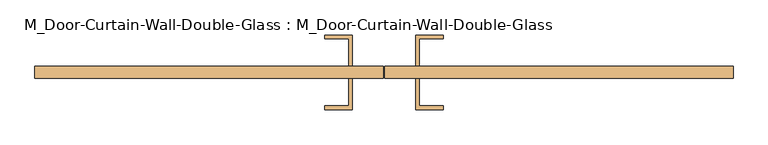
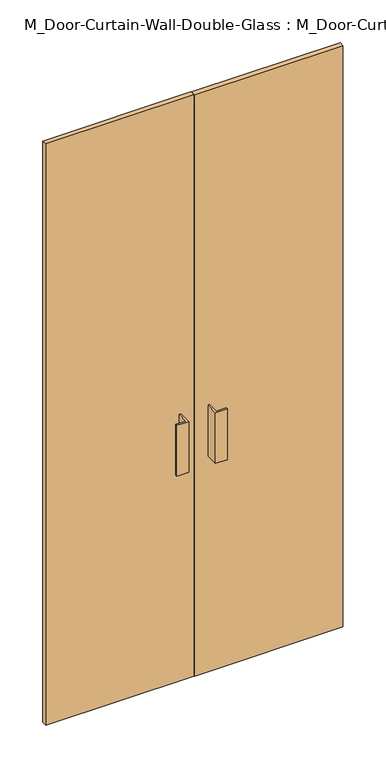
"""IFC4 building model written with IfcOpenShell, lengths in millimetres: door geometry, M_Door-Curtain-Wall-Double-Glass : M_Door-Curtain-Wall-Double-Glass."""

from ifc_helpers import new_model, si_unit, frame, origin, origin_with_axes, place, context, project, spatial, polyline, outline, extrude, source, transform, mapped, element, save


def m_door_curtain_wall_double_glass_m_door_curtain_wall_double_ad7744c8(model_context):
    return source(origin(), model_context, "Body", "SweptSolid", [
        extrude(outline(polyline([(562.5, 31.75), (1.6106001, 31.75), (1.6106001, 50.8), (562.5, 50.8), (562.5, 31.75)])), origin_with_axes(), (0.0, 0.0, 1.0), 2325.0),
        extrude(outline(polyline([(-1.5643999, 31.75), (-562.5, 31.75), (-562.5, 50.8), (-1.5643999, 50.8), (-1.5643999, 31.75)])), origin_with_axes(), (0.0, 0.0, 1.0), 2325.0),
        extrude(outline(polyline([(-50.7768999, 101.6), (-50.7768999, 50.8), (-57.1268999, 50.8), (-57.1268999, 95.25), (-95.2268999, 95.25), (-95.2268999, 101.6), (-50.7768999, 101.6)])), frame((0.0, 0.0, 863.6), z_axis=(0.0, 0.0, 1.0), x_axis=(1.0, 0.0, 0.0)), (0.0, 0.0, 1.0), 203.2),
        extrude(outline(polyline([(50.8231001, 101.6), (95.2731001, 101.6), (95.2731001, 95.25), (57.1731001, 95.25), (57.1731001, 50.8), (50.8231001, 50.8), (50.8231001, 101.6)])), frame((0.0, 0.0, 863.6), z_axis=(0.0, 0.0, 1.0), x_axis=(1.0, 0.0, 0.0)), (0.0, 0.0, 1.0), 203.2),
        extrude(outline(polyline([(-50.7768999, -19.05), (-95.2268999, -19.05), (-95.2268999, -12.7), (-57.1268999, -12.7), (-57.1268999, 31.75), (-50.7768999, 31.75), (-50.7768999, -19.05)])), frame((0.0, 0.0, 863.6), z_axis=(0.0, 0.0, 1.0), x_axis=(1.0, 0.0, 0.0)), (0.0, 0.0, 1.0), 203.2),
        extrude(outline(polyline([(50.8231001, -19.05), (50.8231001, 31.75), (57.1731001, 31.75), (57.1731001, -12.7), (95.2731001, -12.7), (95.2731001, -19.05), (50.8231001, -19.05)])), frame((0.0, 0.0, 863.6), z_axis=(0.0, 0.0, 1.0), x_axis=(1.0, 0.0, 0.0)), (0.0, 0.0, 1.0), 203.2),
    ])


if __name__ == "__main__":
    model = new_model("IFC4")
    model_context = context("Model", 3, world=origin())
    ifc_project = project(units=[si_unit("LENGTHUNIT", "METRE", prefix="MILLI")], contexts=[model_context])
    site = spatial("IfcSite", under=ifc_project)
    building = spatial("IfcBuilding", under=site)
    placement = place(None, origin())
    m_door_curtain_wall_double_glass_m_door_curtain_wall_double_shape = m_door_curtain_wall_double_glass_m_door_curtain_wall_double_ad7744c8(model_context)
    element("IfcDoor", 1, ObjectType="M_Door-Curtain-Wall-Double-Glass : M_Door-Curtain-Wall-Double-Glass", at=placement, inside=building, context=model_context, shape_type="MappedRepresentation", body=[
        mapped(m_door_curtain_wall_double_glass_m_door_curtain_wall_double_shape, transform((0.0, 0.0, 0.0), x_axis=(1.0, 0.0, 0.0), y_axis=(0.0, 1.0, 0.0), z_axis=(0.0, 0.0, 1.0))),
    ])
    save(model, "model.ifc")

# Revit data of these elements
# Type "M_Door-Curtain-Wall-Double-Glass : M_Door-Curtain-Wall-Double-Glass"
#   Type Mark = "47"
#   Assembly Code = "B2030100"
#   Analytic Construction = "<None>"
#   Width [instance default] = 1800 mm
#   Thermal Resistance (R) = 1.7611 (m²·K)/W
#   Swing Angle [instance default] = 90.00°
#   Panel Width [instance default] = 900 mm
#   Offset = 50.8 mm
#   Heat Transfer Coefficient (U) = 0.567826 W/(m²·K)
#   Define Thermal Properties by = 1
#   Function = 1
#   Door Handle Material = Aluminum
#   Glazing = Glass
#   Visual Light Transmittance = 0
#   Solar Heat Gain Coefficient = 0
#   Construction Type Id = ""
# Element 1 (IfcDoor, "M_Door-Curtain-Wall-Double-Glass : M_Door-Curtain-Wall-Double-Glass")
#   Width = 1125 mm
#   Panel Width = 562.5 mm
#   Materials on its faces: "Aluminum", "Glass"
# Materials
#   "Aluminum": class "Metal", colour RGB 136 136 136, transparency 0, Description = "Aluminum 6061", Cost = 0
#   "Glass": class "Glass", colour RGB 245 245 243, transparency 1, Description = "Soda Lime Glass", Cost = 0
